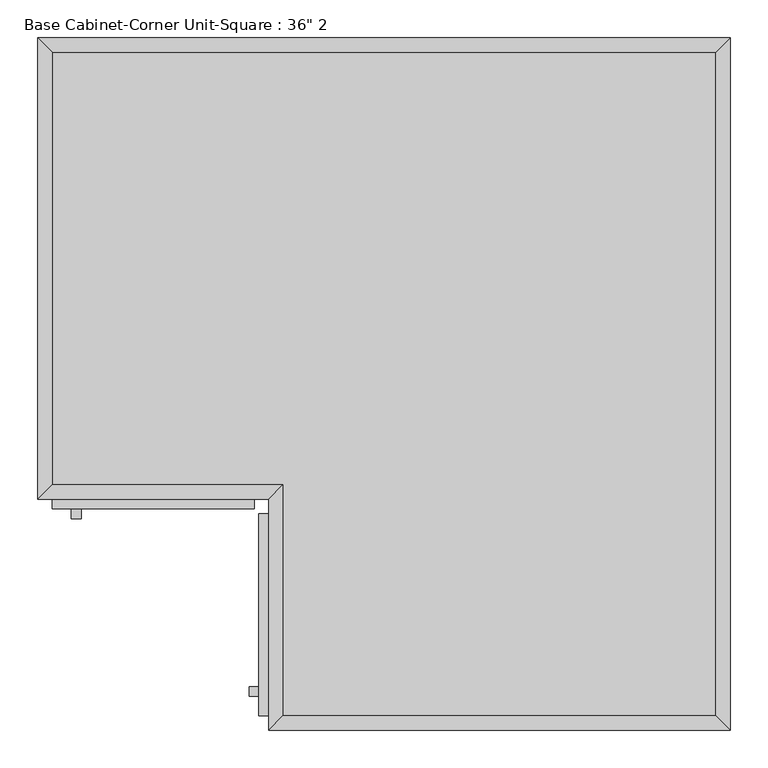
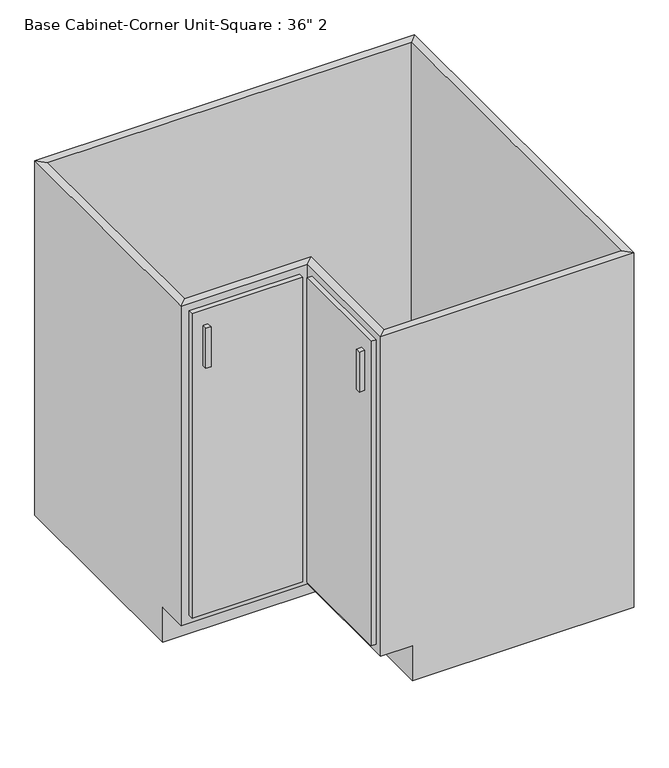
"""IFC4 building model written with IfcOpenShell, lengths in millimetres: furniture geometry."""

from ifc_helpers import new_model, si_unit, frame, origin, place, context, project, spatial, polyline, outline, extrude, faceted_brep, source, transform, mapped, element, save


def furniture_ff3c2f57(model_context):
    return source(origin(), model_context, "Body", "SolidModel", [
        extrude(outline(polyline([(507.6877049, -19.05), (507.6877049, -895.35), (-63.8122951, -895.35), (-63.8122951, -590.55), (-368.6122951, -590.55), (-368.6122951, -19.05), (507.6877049, -19.05)])), frame((0.0, 0.0, 88.9), z_axis=(0.0, 0.0, 1.0), x_axis=(1.0, 0.0, 0.0)), (0.0, 0.0, 1.0), 19.05),
        extrude(outline(polyline([(-101.9122951, -622.3), (-368.6122951, -622.3), (-368.6122951, -609.6), (-101.9122951, -609.6), (-101.9122951, -622.3)])), frame((0.0, 0.0, 107.95), z_axis=(0.0, 0.0, 1.0), x_axis=(1.0, 0.0, 0.0)), (0.0, 0.0, 1.0), 774.7),
        extrude(outline(polyline([(-330.5122951, -635.0), (-343.2122951, -635.0), (-343.2122951, -622.3), (-330.5122951, -622.3), (-330.5122951, -635.0)])), frame((0.0, 0.0, 742.95), z_axis=(0.0, 0.0, 1.0), x_axis=(1.0, 0.0, 0.0)), (0.0, 0.0, 1.0), 101.6),
        extrude(outline(polyline([(-82.8622951, -628.65), (-82.8622951, -895.35), (-95.5622951, -895.35), (-95.5622951, -628.65), (-82.8622951, -628.65)])), frame((0.0, 0.0, 107.95), z_axis=(0.0, 0.0, 1.0), x_axis=(1.0, 0.0, 0.0)), (0.0, 0.0, 1.0), 774.7),
        extrude(outline(polyline([(-95.5622951, -857.25), (-95.5622951, -869.95), (-108.2622951, -869.95), (-108.2622951, -857.25), (-95.5622951, -857.25)])), frame((0.0, 0.0, 742.95), z_axis=(0.0, 0.0, 1.0), x_axis=(1.0, 0.0, 0.0)), (0.0, 0.0, 1.0), 101.6),
        faceted_brep([(-368.6122951, -533.4, 88.9), (-6.6622951, -533.4, 88.9), (-6.6622951, -895.35, 88.9), (507.6877049, -895.35, 88.9), (507.6877049, -19.05, 88.9), (-368.6122951, -19.05, 88.9), (526.7377049, 0.0, 0.0), (526.7377049, -914.4, 0.0), (-6.6622951, -914.4, 0.0), (-6.6622951, -533.4, 0.0), (-387.6622951, -533.4, 0.0), (-387.6622951, 0.0, 0.0), (-387.6622951, 0.0, 901.7), (526.7377049, 0.0, 901.7), (-387.6622951, -533.4, 88.9), (-387.6622951, -609.6, 88.9), (-387.6622951, -609.6, 901.7), (-6.6622951, -914.4, 88.9), (526.7377049, -914.4, 901.7), (-82.8622951, -914.4, 901.7), (-82.8622951, -914.4, 88.9), (507.6877049, -895.35, 901.7), (-63.8122951, -895.35, 88.9), (-63.8122951, -895.35, 901.7), (-63.8122951, -590.55, 88.9), (-63.8122951, -590.55, 901.7), (-82.8622951, -609.6, 901.7), (-82.8622951, -609.6, 88.9), (-368.6122951, -590.55, 88.9), (-368.6122951, -590.55, 901.7), (-368.6122951, -19.05, 901.7), (507.6877049, -19.05, 901.7)], [[[0, 1, 2, 3, 4, 5]], [[6, 7, 8, 9, 10, 11]], [[6, 11, 12, 13]], [[12, 11, 10, 14, 15, 16]], [[10, 9, 1, 0, 14]], [[9, 8, 17, 2, 1]], [[8, 7, 18, 19, 20, 17]], [[18, 7, 6, 13]], [[21, 3, 2, 22, 23]], [[21, 23, 19, 18]], [[20, 22, 2, 17]], [[23, 22, 24, 25]], [[19, 23, 25, 26]], [[20, 19, 26, 27]], [[22, 20, 27, 24]], [[25, 24, 28, 29]], [[26, 25, 29, 16]], [[27, 26, 16, 15]], [[24, 27, 15, 28]], [[29, 28, 0, 5, 30]], [[16, 29, 30, 12]], [[28, 15, 14, 0]], [[30, 5, 4, 31]], [[12, 30, 31, 13]], [[3, 21, 31, 4]], [[21, 18, 13, 31]]]),
    ])


if __name__ == "__main__":
    model = new_model("IFC4")
    model_context = context("Model", 3, world=origin())
    ifc_project = project(units=[si_unit("LENGTHUNIT", "METRE", prefix="MILLI")], contexts=[model_context])
    site = spatial("IfcSite", under=ifc_project)
    building = spatial("IfcBuilding", under=site)
    placement = place(None, origin())
    furniture_shape = furniture_ff3c2f57(model_context)
    element("IfcFurniture", 1, ObjectType="Base Cabinet-Corner Unit-Square : 36\" 2", at=placement, inside=building, context=model_context, shape_type="MappedRepresentation", body=[
        mapped(furniture_shape, transform((0.0, 0.0, 0.0), x_axis=(1.0, 0.0, 0.0), y_axis=(0.0, 1.0, 0.0), z_axis=(0.0, 0.0, 1.0))),
    ])
    save(model, "model.ifc")

# Revit data of these elements
# Type "Base Cabinet-Corner Unit-Square : 36\" 2"
#   Assembly Code = "C1030410"
#   Depth = 2' - 0"
#   Height = 2' - 11 1/2"
#   Toe Depth = 0' - 3"
#   Toe Height = 0' - 3 1/2"
#   Width = 3' - 0"
#   Cabinet Material = Cabinets
#   Door/Drawer Material = Cabinets
#   Handle Material = Cabinets - Handles
#   Default Elevation = 0
# Element 1 (IfcFurniture, "Base Cabinet-Corner Unit-Square : 36\" 2")
#   Materials on its faces: "Cabinets", "Cabinets - Handles"
# Materials
#   "Cabinets": colour RGB 249 249 249, transparency 0
#   "Cabinets - Handles": colour RGB 57 57 57, transparency 0
